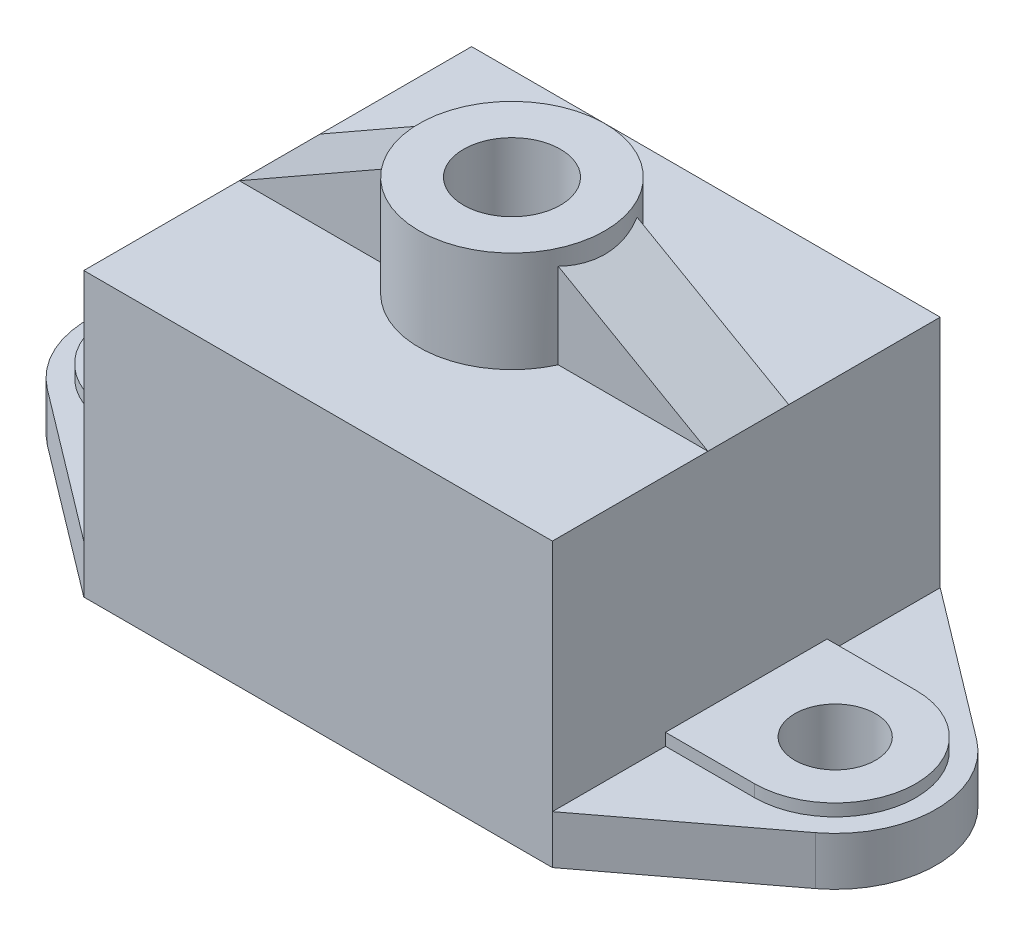
ISO-10303-21;
HEADER;
FILE_DESCRIPTION(('STEP AP214'),'2;1');
FILE_NAME('part.step','',(''),(''),'','','');
FILE_SCHEMA(('AUTOMOTIVE_DESIGN { 1 0 10303 214 1 1 1 1 }'));
ENDSEC;
DATA;
#1=APPLICATION_CONTEXT('core data for automotive mechanical design processes');
#2=APPLICATION_PROTOCOL_DEFINITION('international standard','automotive_design',2000,#1);
#3=PRODUCT_CONTEXT('',#1,'mechanical');
#4=PRODUCT('Part','Part','',(#3));
#5=PRODUCT_RELATED_PRODUCT_CATEGORY('part','',(#4));
#6=PRODUCT_DEFINITION_FORMATION('','',#4);
#7=PRODUCT_DEFINITION_CONTEXT('part definition',#1,'design');
#8=PRODUCT_DEFINITION('design','',#6,#7);
#9=PRODUCT_DEFINITION_SHAPE('','',#8);
#10=(LENGTH_UNIT() NAMED_UNIT(*) SI_UNIT(.MILLI.,.METRE.));
#11=(NAMED_UNIT(*) PLANE_ANGLE_UNIT() SI_UNIT($,.RADIAN.));
#12=(NAMED_UNIT(*) SI_UNIT($,.STERADIAN.) SOLID_ANGLE_UNIT());
#13=UNCERTAINTY_MEASURE_WITH_UNIT(LENGTH_MEASURE(1.E-05),#10,'distance_accuracy_value','');
#14=(GEOMETRIC_REPRESENTATION_CONTEXT(3) GLOBAL_UNCERTAINTY_ASSIGNED_CONTEXT((#13)) GLOBAL_UNIT_ASSIGNED_CONTEXT((#10,
#11,#12)) REPRESENTATION_CONTEXT('',''));
#15=CARTESIAN_POINT('',(0.,0.,0.));
#16=DIRECTION('',(0.,0.,1.));
#17=DIRECTION('',(1.,0.,0.));
#18=AXIS2_PLACEMENT_3D('',#15,#16,#17);
#19=CARTESIAN_POINT('',(116.,70.,96.));
#20=DIRECTION('',(0.,-1.,0.));
#21=DIRECTION('',(0.,0.,-1.));
#22=AXIS2_PLACEMENT_3D('',#19,#20,#21);
#23=PLANE('',#22);
#24=DIRECTION('',(-1.,0.,0.));
#25=VECTOR('',#24,1.);
#26=CARTESIAN_POINT('',(35.,70.,57.5));
#27=LINE('',#26,#25);
#28=CARTESIAN_POINT('',(37.0536399343466,70.,57.5));
#29=VERTEX_POINT('',#28);
#30=CARTESIAN_POINT('',(0.,70.,57.5));
#31=VERTEX_POINT('',#30);
#32=EDGE_CURVE('E208',#29,#31,#27,.T.);
#33=ORIENTED_EDGE('',*,*,#32,.T.);
#34=DIRECTION('',(0.,0.,-1.));
#35=VECTOR('',#34,1.);
#36=CARTESIAN_POINT('',(0.,70.,96.));
#37=LINE('',#36,#35);
#38=CARTESIAN_POINT('',(0.,70.,96.));
#39=VERTEX_POINT('',#38);
#40=EDGE_CURVE('E224',#39,#31,#37,.T.);
#41=ORIENTED_EDGE('',*,*,#40,.F.);
#42=DIRECTION('',(-1.,0.,0.));
#43=VECTOR('',#42,1.);
#44=CARTESIAN_POINT('',(116.,70.,96.));
#45=LINE('',#44,#43);
#46=CARTESIAN_POINT('',(116.,70.,96.));
#47=VERTEX_POINT('',#46);
#48=EDGE_CURVE('E232',#47,#39,#45,.T.);
#49=ORIENTED_EDGE('',*,*,#48,.F.);
#50=DIRECTION('',(0.,0.,-1.));
#51=VECTOR('',#50,1.);
#52=CARTESIAN_POINT('',(116.,70.,96.));
#53=LINE('',#52,#51);
#54=CARTESIAN_POINT('',(116.,70.,57.5));
#55=VERTEX_POINT('',#54);
#56=EDGE_CURVE('E231',#47,#55,#53,.T.);
#57=ORIENTED_EDGE('',*,*,#56,.T.);
#58=DIRECTION('',(1.,0.,0.));
#59=VECTOR('',#58,1.);
#60=CARTESIAN_POINT('',(81.,70.,57.5));
#61=LINE('',#60,#59);
#62=CARTESIAN_POINT('',(78.9463600656534,70.,57.5));
#63=VERTEX_POINT('',#62);
#64=EDGE_CURVE('E259',#63,#55,#61,.T.);
#65=ORIENTED_EDGE('',*,*,#64,.F.);
#66=CARTESIAN_POINT('',(58.,70.,48.));
#67=DIRECTION('',(0.,-1.,0.));
#68=DIRECTION('',(0.,0.,-1.));
#69=AXIS2_PLACEMENT_3D('',#66,#67,#68);
#70=CIRCLE('',#69,23.);
#71=EDGE_CURVE('E228',#29,#63,#70,.F.);
#72=ORIENTED_EDGE('',*,*,#71,.F.);
#73=EDGE_LOOP('',(#33,#41,#49,#57,#65,#72));
#74=FACE_BOUND('',#73,.T.);
#75=ADVANCED_FACE('F41',(#74),#23,.F.);
#76=CARTESIAN_POINT('',(58.,95.,48.));
#77=DIRECTION('',(0.,-1.,0.));
#78=DIRECTION('',(0.,0.,-1.));
#79=AXIS2_PLACEMENT_3D('',#76,#77,#78);
#80=CYLINDRICAL_SURFACE('',#79,23.);
#81=CARTESIAN_POINT('',(58.,95.,48.));
#82=DIRECTION('',(0.,1.,0.));
#83=DIRECTION('',(0.,0.,1.));
#84=AXIS2_PLACEMENT_3D('',#81,#82,#83);
#85=CIRCLE('',#84,23.);
#86=CARTESIAN_POINT('',(58.,95.,71.));
#87=VERTEX_POINT('',#86);
#88=EDGE_CURVE('E277',#87,#87,#85,.T.);
#89=ORIENTED_EDGE('',*,*,#88,.F.);
#90=EDGE_LOOP('',(#89));
#91=FACE_BOUND('',#90,.T.);
#92=DIRECTION('',(0.,-1.,0.));
#93=VECTOR('',#92,1.);
#94=CARTESIAN_POINT('',(37.0536399343466,95.,57.5));
#95=LINE('',#94,#93);
#96=CARTESIAN_POINT('',(37.0536399343466,91.128111029422,57.5));
#97=VERTEX_POINT('',#96);
#98=EDGE_CURVE('E216',#29,#97,#95,.F.);
#99=ORIENTED_EDGE('',*,*,#98,.F.);
#100=ORIENTED_EDGE('',*,*,#71,.T.);
#101=DIRECTION('',(0.,-1.,0.));
#102=VECTOR('',#101,1.);
#103=CARTESIAN_POINT('',(78.9463600656534,95.,57.5));
#104=LINE('',#103,#102);
#105=CARTESIAN_POINT('',(78.9463600656534,91.1281110294221,57.5));
#106=VERTEX_POINT('',#105);
#107=EDGE_CURVE('E11',#106,#63,#104,.T.);
#108=ORIENTED_EDGE('',*,*,#107,.F.);
#109=CARTESIAN_POINT('',(58.,103.071796505762,48.));
#110=DIRECTION('',(-0.495336394229628,-0.868701247007043,0.));
#111=DIRECTION('',(0.868701247007043,-0.495336394229628,0.));
#112=AXIS2_PLACEMENT_3D('',#109,#110,#111);
#113=ELLIPSE('',#112,26.4763059558651,23.);
#114=CARTESIAN_POINT('',(78.4633819296811,91.4035067988981,37.5));
#115=VERTEX_POINT('',#114);
#116=EDGE_CURVE('E47',#115,#106,#113,.T.);
#117=ORIENTED_EDGE('',*,*,#116,.F.);
#118=DIRECTION('',(0.,-1.,0.));
#119=VECTOR('',#118,1.);
#120=CARTESIAN_POINT('',(78.4633819296811,95.,37.5));
#121=LINE('',#120,#119);
#122=CARTESIAN_POINT('',(78.4633819296811,70.,37.5));
#123=VERTEX_POINT('',#122);
#124=EDGE_CURVE('E242',#115,#123,#121,.T.);
#125=ORIENTED_EDGE('',*,*,#124,.T.);
#126=CARTESIAN_POINT('',(37.5366180703189,70.,37.5));
#127=VERTEX_POINT('',#126);
#128=EDGE_CURVE('E241',#123,#127,#70,.F.);
#129=ORIENTED_EDGE('',*,*,#128,.T.);
#130=DIRECTION('',(0.,-1.,0.));
#131=VECTOR('',#130,1.);
#132=CARTESIAN_POINT('',(37.5366180703189,95.,37.5));
#133=LINE('',#132,#131);
#134=CARTESIAN_POINT('',(37.5366180703189,91.403506798898,37.5));
#135=VERTEX_POINT('',#134);
#136=EDGE_CURVE('E209',#127,#135,#133,.F.);
#137=ORIENTED_EDGE('',*,*,#136,.T.);
#138=CARTESIAN_POINT('',(58.,103.071796505762,48.));
#139=DIRECTION('',(-0.495336394229628,0.868701247007043,0.));
#140=DIRECTION('',(-0.868701247007043,-0.495336394229628,0.));
#141=AXIS2_PLACEMENT_3D('',#138,#139,#140);
#142=ELLIPSE('',#141,26.4763059558651,23.);
#143=EDGE_CURVE('E265',#135,#97,#142,.T.);
#144=ORIENTED_EDGE('',*,*,#143,.T.);
#145=EDGE_LOOP('',(#99,#100,#108,#117,#125,#129,#137,#144));
#146=FACE_BOUND('',#145,.T.);
#147=ADVANCED_FACE('F258',(#91,#146),#80,.T.);
#148=CARTESIAN_POINT('',(0.,70.,37.5));
#149=VERTEX_POINT('',#148);
#150=CARTESIAN_POINT('',(0.,70.,0.));
#151=VERTEX_POINT('',#150);
#152=EDGE_CURVE('E233',#149,#151,#37,.T.);
#153=ORIENTED_EDGE('',*,*,#152,.F.);
#154=DIRECTION('',(-1.,0.,0.));
#155=VECTOR('',#154,1.);
#156=CARTESIAN_POINT('',(35.,70.,37.5));
#157=LINE('',#156,#155);
#158=EDGE_CURVE('E220',#127,#149,#157,.T.);
#159=ORIENTED_EDGE('',*,*,#158,.F.);
#160=ORIENTED_EDGE('',*,*,#128,.F.);
#161=DIRECTION('',(1.,0.,0.));
#162=VECTOR('',#161,1.);
#163=CARTESIAN_POINT('',(81.,70.,37.5));
#164=LINE('',#163,#162);
#165=CARTESIAN_POINT('',(116.,70.,37.5));
#166=VERTEX_POINT('',#165);
#167=EDGE_CURVE('E61',#123,#166,#164,.T.);
#168=ORIENTED_EDGE('',*,*,#167,.T.);
#169=CARTESIAN_POINT('',(116.,70.,0.));
#170=VERTEX_POINT('',#169);
#171=EDGE_CURVE('E229',#166,#170,#53,.T.);
#172=ORIENTED_EDGE('',*,*,#171,.T.);
#173=DIRECTION('',(-1.,0.,0.));
#174=VECTOR('',#173,1.);
#175=CARTESIAN_POINT('',(116.,70.,0.));
#176=LINE('',#175,#174);
#177=EDGE_CURVE('E240',#170,#151,#176,.T.);
#178=ORIENTED_EDGE('',*,*,#177,.T.);
#179=EDGE_LOOP('',(#153,#159,#160,#168,#172,#178));
#180=FACE_BOUND('',#179,.T.);
#181=ADVANCED_FACE('F432',(#180),#23,.F.);
#182=CARTESIAN_POINT('',(116.,0.,96.));
#183=DIRECTION('',(-1.,0.,0.));
#184=DIRECTION('',(0.,0.,1.));
#185=AXIS2_PLACEMENT_3D('',#182,#183,#184);
#186=PLANE('',#185);
#187=DIRECTION('',(0.,-1.,0.));
#188=VECTOR('',#187,1.);
#189=CARTESIAN_POINT('',(116.,15.,28.));
#190=LINE('',#189,#188);
#191=CARTESIAN_POINT('',(116.,15.,28.));
#192=VERTEX_POINT('',#191);
#193=CARTESIAN_POINT('',(116.,12.,28.));
#194=VERTEX_POINT('',#193);
#195=EDGE_CURVE('E373',#192,#194,#190,.T.);
#196=ORIENTED_EDGE('',*,*,#195,.T.);
#197=DIRECTION('',(0.,0.,1.));
#198=VECTOR('',#197,1.);
#199=CARTESIAN_POINT('',(116.,12.,0.));
#200=LINE('',#199,#198);
#201=CARTESIAN_POINT('',(116.,12.,0.));
#202=VERTEX_POINT('',#201);
#203=EDGE_CURVE('E390',#202,#194,#200,.T.);
#204=ORIENTED_EDGE('',*,*,#203,.F.);
#205=DIRECTION('',(0.,1.,0.));
#206=VECTOR('',#205,1.);
#207=CARTESIAN_POINT('',(116.,0.,0.));
#208=LINE('',#207,#206);
#209=EDGE_CURVE('E416',#202,#170,#208,.T.);
#210=ORIENTED_EDGE('',*,*,#209,.T.);
#211=ORIENTED_EDGE('',*,*,#171,.F.);
#212=DIRECTION('',(0.,0.,-1.));
#213=VECTOR('',#212,1.);
#214=CARTESIAN_POINT('',(116.,70.,57.5));
#215=LINE('',#214,#213);
#216=EDGE_CURVE('E269',#55,#166,#215,.T.);
#217=ORIENTED_EDGE('',*,*,#216,.F.);
#218=ORIENTED_EDGE('',*,*,#56,.F.);
#219=DIRECTION('',(0.,1.,0.));
#220=VECTOR('',#219,1.);
#221=CARTESIAN_POINT('',(116.,0.,96.));
#222=LINE('',#221,#220);
#223=CARTESIAN_POINT('',(116.,12.,96.));
#224=VERTEX_POINT('',#223);
#225=EDGE_CURVE('E409',#224,#47,#222,.T.);
#226=ORIENTED_EDGE('',*,*,#225,.F.);
#227=CARTESIAN_POINT('',(116.,12.,68.));
#228=VERTEX_POINT('',#227);
#229=EDGE_CURVE('E387',#228,#224,#200,.T.);
#230=ORIENTED_EDGE('',*,*,#229,.F.);
#231=DIRECTION('',(0.,-1.,0.));
#232=VECTOR('',#231,1.);
#233=CARTESIAN_POINT('',(116.,15.,68.));
#234=LINE('',#233,#232);
#235=CARTESIAN_POINT('',(116.,15.,68.));
#236=VERTEX_POINT('',#235);
#237=EDGE_CURVE('E371',#236,#228,#234,.T.);
#238=ORIENTED_EDGE('',*,*,#237,.F.);
#239=DIRECTION('',(0.,0.,1.));
#240=VECTOR('',#239,1.);
#241=CARTESIAN_POINT('',(116.,15.,28.));
#242=LINE('',#241,#240);
#243=EDGE_CURVE('E360',#192,#236,#242,.T.);
#244=ORIENTED_EDGE('',*,*,#243,.F.);
#245=EDGE_LOOP('',(#196,#204,#210,#211,#217,#218,#226,#230,#238,#244));
#246=FACE_BOUND('',#245,.T.);
#247=ADVANCED_FACE('F430',(#246),#186,.F.);
#248=CARTESIAN_POINT('',(138.,12.,48.));
#249=DIRECTION('',(0.,1.,0.));
#250=DIRECTION('',(0.,0.,1.));
#251=AXIS2_PLACEMENT_3D('',#248,#249,#250);
#252=PLANE('',#251);
#253=ORIENTED_EDGE('',*,*,#203,.T.);
#254=DIRECTION('',(-1.,0.,0.));
#255=VECTOR('',#254,1.);
#256=CARTESIAN_POINT('',(138.,12.,28.));
#257=LINE('',#256,#255);
#258=CARTESIAN_POINT('',(138.,12.,28.));
#259=VERTEX_POINT('',#258);
#260=EDGE_CURVE('E366',#259,#194,#257,.T.);
#261=ORIENTED_EDGE('',*,*,#260,.F.);
#262=CARTESIAN_POINT('',(138.,12.,48.));
#263=DIRECTION('',(0.,1.,0.));
#264=DIRECTION('',(0.,0.,1.));
#265=AXIS2_PLACEMENT_3D('',#262,#263,#264);
#266=CIRCLE('',#265,20.);
#267=CARTESIAN_POINT('',(138.,12.,68.));
#268=VERTEX_POINT('',#267);
#269=EDGE_CURVE('E349',#268,#259,#266,.T.);
#270=ORIENTED_EDGE('',*,*,#269,.F.);
#271=DIRECTION('',(1.,0.,0.));
#272=VECTOR('',#271,1.);
#273=CARTESIAN_POINT('',(116.,12.,68.));
#274=LINE('',#273,#272);
#275=EDGE_CURVE('E357',#228,#268,#274,.T.);
#276=ORIENTED_EDGE('',*,*,#275,.F.);
#277=ORIENTED_EDGE('',*,*,#229,.T.);
#278=DIRECTION('',(0.797409398842377,0.,-0.603438688383367));
#279=VECTOR('',#278,1.);
#280=CARTESIAN_POINT('',(116.,12.,96.));
#281=LINE('',#280,#279);
#282=CARTESIAN_POINT('',(153.085967209584,12.,67.9352349710594));
#283=VERTEX_POINT('',#282);
#284=EDGE_CURVE('E388',#224,#283,#281,.T.);
#285=ORIENTED_EDGE('',*,*,#284,.T.);
#286=CARTESIAN_POINT('',(138.,12.,48.));
#287=DIRECTION('',(0.,1.,0.));
#288=DIRECTION('',(0.,0.,1.));
#289=AXIS2_PLACEMENT_3D('',#286,#287,#288);
#290=CIRCLE('',#289,25.);
#291=CARTESIAN_POINT('',(153.085967209584,12.,28.0647650289406));
#292=VERTEX_POINT('',#291);
#293=EDGE_CURVE('E378',#283,#292,#290,.T.);
#294=ORIENTED_EDGE('',*,*,#293,.T.);
#295=DIRECTION('',(-0.797409398842377,0.,-0.603438688383367));
#296=VECTOR('',#295,1.);
#297=CARTESIAN_POINT('',(116.,12.,0.));
#298=LINE('',#297,#296);
#299=EDGE_CURVE('E385',#292,#202,#298,.T.);
#300=ORIENTED_EDGE('',*,*,#299,.T.);
#301=EDGE_LOOP('',(#253,#261,#270,#276,#277,#285,#294,#300));
#302=FACE_BOUND('',#301,.T.);
#303=ADVANCED_FACE('F463',(#302),#252,.T.);
#304=CARTESIAN_POINT('',(0.,70.,96.));
#305=DIRECTION('',(1.,0.,0.));
#306=DIRECTION('',(0.,0.,-1.));
#307=AXIS2_PLACEMENT_3D('',#304,#305,#306);
#308=PLANE('',#307);
#309=DIRECTION('',(0.,0.,1.));
#310=VECTOR('',#309,1.);
#311=CARTESIAN_POINT('',(0.,15.,28.));
#312=LINE('',#311,#310);
#313=CARTESIAN_POINT('',(0.,15.,28.));
#314=VERTEX_POINT('',#313);
#315=CARTESIAN_POINT('',(0.,15.,68.));
#316=VERTEX_POINT('',#315);
#317=EDGE_CURVE('E294',#314,#316,#312,.T.);
#318=ORIENTED_EDGE('',*,*,#317,.T.);
#319=DIRECTION('',(0.,-1.,0.));
#320=VECTOR('',#319,1.);
#321=CARTESIAN_POINT('',(0.,15.,68.));
#322=LINE('',#321,#320);
#323=CARTESIAN_POINT('',(0.,12.,68.));
#324=VERTEX_POINT('',#323);
#325=EDGE_CURVE('E309',#316,#324,#322,.T.);
#326=ORIENTED_EDGE('',*,*,#325,.T.);
#327=DIRECTION('',(0.,0.,1.));
#328=VECTOR('',#327,1.);
#329=CARTESIAN_POINT('',(0.,12.,0.));
#330=LINE('',#329,#328);
#331=CARTESIAN_POINT('',(0.,12.,96.));
#332=VERTEX_POINT('',#331);
#333=EDGE_CURVE('E324',#324,#332,#330,.T.);
#334=ORIENTED_EDGE('',*,*,#333,.T.);
#335=DIRECTION('',(0.,-1.,0.));
#336=VECTOR('',#335,1.);
#337=CARTESIAN_POINT('',(0.,70.,96.));
#338=LINE('',#337,#336);
#339=EDGE_CURVE('E230',#39,#332,#338,.T.);
#340=ORIENTED_EDGE('',*,*,#339,.F.);
#341=ORIENTED_EDGE('',*,*,#40,.T.);
#342=DIRECTION('',(0.,0.,-1.));
#343=VECTOR('',#342,1.);
#344=CARTESIAN_POINT('',(0.,70.,57.5));
#345=LINE('',#344,#343);
#346=EDGE_CURVE('E202',#31,#149,#345,.T.);
#347=ORIENTED_EDGE('',*,*,#346,.T.);
#348=ORIENTED_EDGE('',*,*,#152,.T.);
#349=DIRECTION('',(0.,-1.,0.));
#350=VECTOR('',#349,1.);
#351=CARTESIAN_POINT('',(0.,70.,0.));
#352=LINE('',#351,#350);
#353=CARTESIAN_POINT('',(0.,12.,0.));
#354=VERTEX_POINT('',#353);
#355=EDGE_CURVE('E404',#151,#354,#352,.T.);
#356=ORIENTED_EDGE('',*,*,#355,.T.);
#357=CARTESIAN_POINT('',(0.,12.,28.));
#358=VERTEX_POINT('',#357);
#359=EDGE_CURVE('E321',#354,#358,#330,.T.);
#360=ORIENTED_EDGE('',*,*,#359,.T.);
#361=DIRECTION('',(0.,-1.,0.));
#362=VECTOR('',#361,1.);
#363=CARTESIAN_POINT('',(0.,15.,28.));
#364=LINE('',#363,#362);
#365=EDGE_CURVE('E310',#314,#358,#364,.T.);
#366=ORIENTED_EDGE('',*,*,#365,.F.);
#367=EDGE_LOOP('',(#318,#326,#334,#340,#341,#347,#348,#356,#360,#366));
#368=FACE_BOUND('',#367,.T.);
#369=ADVANCED_FACE('F43',(#368),#308,.F.);
#370=CARTESIAN_POINT('',(0.,0.,96.));
#371=DIRECTION('',(0.,1.,0.));
#372=DIRECTION('',(0.,0.,1.));
#373=AXIS2_PLACEMENT_3D('',#370,#371,#372);
#374=PLANE('',#373);
#375=CARTESIAN_POINT('',(-22.,0.,48.));
#376=DIRECTION('',(0.,-1.,0.));
#377=DIRECTION('',(0.,0.,1.));
#378=AXIS2_PLACEMENT_3D('',#375,#376,#377);
#379=CIRCLE('',#378,10.);
#380=CARTESIAN_POINT('',(-22.,0.,58.));
#381=VERTEX_POINT('',#380);
#382=EDGE_CURVE('E285',#381,#381,#379,.T.);
#383=ORIENTED_EDGE('',*,*,#382,.F.);
#384=EDGE_LOOP('',(#383));
#385=FACE_BOUND('',#384,.T.);
#386=CARTESIAN_POINT('',(138.,0.,48.));
#387=DIRECTION('',(0.,1.,0.));
#388=DIRECTION('',(0.,0.,1.));
#389=AXIS2_PLACEMENT_3D('',#386,#387,#388);
#390=CIRCLE('',#389,10.);
#391=CARTESIAN_POINT('',(138.,0.,58.));
#392=VERTEX_POINT('',#391);
#393=EDGE_CURVE('E350',#392,#392,#390,.T.);
#394=ORIENTED_EDGE('',*,*,#393,.T.);
#395=EDGE_LOOP('',(#394));
#396=FACE_BOUND('',#395,.T.);
#397=DIRECTION('',(1.,0.,0.));
#398=VECTOR('',#397,1.);
#399=CARTESIAN_POINT('',(0.,0.,0.));
#400=LINE('',#399,#398);
#401=CARTESIAN_POINT('',(0.,0.,0.));
#402=VERTEX_POINT('',#401);
#403=CARTESIAN_POINT('',(116.,0.,0.));
#404=VERTEX_POINT('',#403);
#405=EDGE_CURVE('E414',#402,#404,#400,.T.);
#406=ORIENTED_EDGE('',*,*,#405,.T.);
#407=DIRECTION('',(-0.797409398842377,0.,-0.603438688383367));
#408=VECTOR('',#407,1.);
#409=CARTESIAN_POINT('',(116.,0.,0.));
#410=LINE('',#409,#408);
#411=CARTESIAN_POINT('',(153.085967209584,0.,28.0647650289406));
#412=VERTEX_POINT('',#411);
#413=EDGE_CURVE('E394',#412,#404,#410,.T.);
#414=ORIENTED_EDGE('',*,*,#413,.F.);
#415=CARTESIAN_POINT('',(138.,0.,48.));
#416=DIRECTION('',(0.,1.,0.));
#417=DIRECTION('',(0.,0.,1.));
#418=AXIS2_PLACEMENT_3D('',#415,#416,#417);
#419=CIRCLE('',#418,25.);
#420=CARTESIAN_POINT('',(153.085967209584,0.,67.9352349710594));
#421=VERTEX_POINT('',#420);
#422=EDGE_CURVE('E377',#421,#412,#419,.T.);
#423=ORIENTED_EDGE('',*,*,#422,.F.);
#424=DIRECTION('',(0.797409398842377,0.,-0.603438688383367));
#425=VECTOR('',#424,1.);
#426=CARTESIAN_POINT('',(116.,0.,96.));
#427=LINE('',#426,#425);
#428=CARTESIAN_POINT('',(116.,0.,96.));
#429=VERTEX_POINT('',#428);
#430=EDGE_CURVE('E384',#429,#421,#427,.T.);
#431=ORIENTED_EDGE('',*,*,#430,.F.);
#432=DIRECTION('',(1.,0.,0.));
#433=VECTOR('',#432,1.);
#434=CARTESIAN_POINT('',(0.,0.,96.));
#435=LINE('',#434,#433);
#436=CARTESIAN_POINT('',(0.,0.,96.));
#437=VERTEX_POINT('',#436);
#438=EDGE_CURVE('E407',#437,#429,#435,.T.);
#439=ORIENTED_EDGE('',*,*,#438,.F.);
#440=DIRECTION('',(-0.797409398842377,0.,-0.603438688383367));
#441=VECTOR('',#440,1.);
#442=CARTESIAN_POINT('',(0.,0.,96.));
#443=LINE('',#442,#441);
#444=CARTESIAN_POINT('',(-37.0859672095842,0.,67.9352349710594));
#445=VERTEX_POINT('',#444);
#446=EDGE_CURVE('E334',#437,#445,#443,.T.);
#447=ORIENTED_EDGE('',*,*,#446,.T.);
#448=CARTESIAN_POINT('',(-22.,0.,48.));
#449=DIRECTION('',(0.,-1.,0.));
#450=DIRECTION('',(0.,0.,1.));
#451=AXIS2_PLACEMENT_3D('',#448,#449,#450);
#452=CIRCLE('',#451,25.);
#453=CARTESIAN_POINT('',(-37.0859672095842,0.,28.0647650289406));
#454=VERTEX_POINT('',#453);
#455=EDGE_CURVE('E314',#445,#454,#452,.T.);
#456=ORIENTED_EDGE('',*,*,#455,.T.);
#457=DIRECTION('',(0.797409398842377,0.,-0.603438688383367));
#458=VECTOR('',#457,1.);
#459=CARTESIAN_POINT('',(0.,0.,0.));
#460=LINE('',#459,#458);
#461=EDGE_CURVE('E318',#454,#402,#460,.T.);
#462=ORIENTED_EDGE('',*,*,#461,.T.);
#463=EDGE_LOOP('',(#406,#414,#423,#431,#439,#447,#456,#462));
#464=FACE_BOUND('',#463,.T.);
#465=ADVANCED_FACE('F468',(#385,#396,#464),#374,.F.);
#466=CARTESIAN_POINT('',(0.,0.,96.));
#467=DIRECTION('',(0.,0.,1.));
#468=DIRECTION('',(1.,0.,0.));
#469=AXIS2_PLACEMENT_3D('',#466,#467,#468);
#470=PLANE('',#469);
#471=ORIENTED_EDGE('',*,*,#339,.T.);
#472=DIRECTION('',(0.,-1.,0.));
#473=VECTOR('',#472,1.);
#474=CARTESIAN_POINT('',(0.,12.,96.));
#475=LINE('',#474,#473);
#476=EDGE_CURVE('E342',#332,#437,#475,.T.);
#477=ORIENTED_EDGE('',*,*,#476,.T.);
#478=ORIENTED_EDGE('',*,*,#438,.T.);
#479=EDGE_CURVE('E406',#429,#224,#222,.T.);
#480=ORIENTED_EDGE('',*,*,#479,.T.);
#481=ORIENTED_EDGE('',*,*,#225,.T.);
#482=ORIENTED_EDGE('',*,*,#48,.T.);
#483=EDGE_LOOP('',(#471,#477,#478,#480,#481,#482));
#484=FACE_BOUND('',#483,.T.);
#485=ADVANCED_FACE('F475',(#484),#470,.T.);
#486=CARTESIAN_POINT('',(0.,0.,0.));
#487=DIRECTION('',(0.,0.,1.));
#488=DIRECTION('',(1.,0.,0.));
#489=AXIS2_PLACEMENT_3D('',#486,#487,#488);
#490=PLANE('',#489);
#491=ORIENTED_EDGE('',*,*,#355,.F.);
#492=ORIENTED_EDGE('',*,*,#177,.F.);
#493=ORIENTED_EDGE('',*,*,#209,.F.);
#494=EDGE_CURVE('E417',#404,#202,#208,.T.);
#495=ORIENTED_EDGE('',*,*,#494,.F.);
#496=ORIENTED_EDGE('',*,*,#405,.F.);
#497=DIRECTION('',(0.,-1.,0.));
#498=VECTOR('',#497,1.);
#499=CARTESIAN_POINT('',(0.,12.,0.));
#500=LINE('',#499,#498);
#501=EDGE_CURVE('E339',#354,#402,#500,.T.);
#502=ORIENTED_EDGE('',*,*,#501,.F.);
#503=EDGE_LOOP('',(#491,#492,#493,#495,#496,#502));
#504=FACE_BOUND('',#503,.T.);
#505=ADVANCED_FACE('F427',(#504),#490,.F.);
#506=CARTESIAN_POINT('',(138.,12.,48.));
#507=DIRECTION('',(0.,-1.,0.));
#508=DIRECTION('',(0.,0.,-1.));
#509=AXIS2_PLACEMENT_3D('',#506,#507,#508);
#510=CYLINDRICAL_SURFACE('',#509,25.);
#511=ORIENTED_EDGE('',*,*,#422,.T.);
#512=DIRECTION('',(0.,-1.,0.));
#513=VECTOR('',#512,1.);
#514=CARTESIAN_POINT('',(153.085967209584,12.,28.0647650289406));
#515=LINE('',#514,#513);
#516=EDGE_CURVE('E402',#292,#412,#515,.T.);
#517=ORIENTED_EDGE('',*,*,#516,.F.);
#518=ORIENTED_EDGE('',*,*,#293,.F.);
#519=DIRECTION('',(0.,-1.,0.));
#520=VECTOR('',#519,1.);
#521=CARTESIAN_POINT('',(153.085967209584,12.,67.9352349710594));
#522=LINE('',#521,#520);
#523=EDGE_CURVE('E395',#283,#421,#522,.T.);
#524=ORIENTED_EDGE('',*,*,#523,.T.);
#525=EDGE_LOOP('',(#511,#517,#518,#524));
#526=FACE_BOUND('',#525,.T.);
#527=ADVANCED_FACE('F493',(#526),#510,.T.);
#528=CARTESIAN_POINT('',(116.,12.,0.));
#529=DIRECTION('',(-0.603438688383367,0.,0.797409398842377));
#530=DIRECTION('',(0.797409398842377,0.,0.603438688383367));
#531=AXIS2_PLACEMENT_3D('',#528,#529,#530);
#532=PLANE('',#531);
#533=ORIENTED_EDGE('',*,*,#413,.T.);
#534=ORIENTED_EDGE('',*,*,#494,.T.);
#535=ORIENTED_EDGE('',*,*,#299,.F.);
#536=ORIENTED_EDGE('',*,*,#516,.T.);
#537=EDGE_LOOP('',(#533,#534,#535,#536));
#538=FACE_BOUND('',#537,.T.);
#539=ADVANCED_FACE('F487',(#538),#532,.F.);
#540=CARTESIAN_POINT('',(116.,12.,96.));
#541=DIRECTION('',(-0.603438688383367,0.,-0.797409398842377));
#542=DIRECTION('',(-0.797409398842377,0.,0.603438688383367));
#543=AXIS2_PLACEMENT_3D('',#540,#541,#542);
#544=PLANE('',#543);
#545=ORIENTED_EDGE('',*,*,#430,.T.);
#546=ORIENTED_EDGE('',*,*,#523,.F.);
#547=ORIENTED_EDGE('',*,*,#284,.F.);
#548=ORIENTED_EDGE('',*,*,#479,.F.);
#549=EDGE_LOOP('',(#545,#546,#547,#548));
#550=FACE_BOUND('',#549,.T.);
#551=ADVANCED_FACE('F500',(#550),#544,.F.);
#552=CARTESIAN_POINT('',(138.,15.,48.));
#553=DIRECTION('',(0.,-1.,0.));
#554=DIRECTION('',(0.,0.,-1.));
#555=AXIS2_PLACEMENT_3D('',#552,#553,#554);
#556=CYLINDRICAL_SURFACE('',#555,20.);
#557=ORIENTED_EDGE('',*,*,#269,.T.);
#558=DIRECTION('',(0.,-1.,0.));
#559=VECTOR('',#558,1.);
#560=CARTESIAN_POINT('',(138.,15.,28.));
#561=LINE('',#560,#559);
#562=CARTESIAN_POINT('',(138.,15.,28.));
#563=VERTEX_POINT('',#562);
#564=EDGE_CURVE('E376',#563,#259,#561,.T.);
#565=ORIENTED_EDGE('',*,*,#564,.F.);
#566=CARTESIAN_POINT('',(138.,15.,48.));
#567=DIRECTION('',(0.,1.,0.));
#568=DIRECTION('',(0.,0.,1.));
#569=AXIS2_PLACEMENT_3D('',#566,#567,#568);
#570=CIRCLE('',#569,20.);
#571=CARTESIAN_POINT('',(138.,15.,68.));
#572=VERTEX_POINT('',#571);
#573=EDGE_CURVE('E354',#572,#563,#570,.T.);
#574=ORIENTED_EDGE('',*,*,#573,.F.);
#575=DIRECTION('',(0.,-1.,0.));
#576=VECTOR('',#575,1.);
#577=CARTESIAN_POINT('',(138.,15.,68.));
#578=LINE('',#577,#576);
#579=EDGE_CURVE('E361',#572,#268,#578,.T.);
#580=ORIENTED_EDGE('',*,*,#579,.T.);
#581=EDGE_LOOP('',(#557,#565,#574,#580));
#582=FACE_BOUND('',#581,.T.);
#583=ADVANCED_FACE('F555',(#582),#556,.T.);
#584=CARTESIAN_POINT('',(138.,15.,28.));
#585=DIRECTION('',(0.,0.,1.));
#586=DIRECTION('',(1.,0.,0.));
#587=AXIS2_PLACEMENT_3D('',#584,#585,#586);
#588=PLANE('',#587);
#589=ORIENTED_EDGE('',*,*,#260,.T.);
#590=ORIENTED_EDGE('',*,*,#195,.F.);
#591=DIRECTION('',(-1.,0.,0.));
#592=VECTOR('',#591,1.);
#593=CARTESIAN_POINT('',(138.,15.,28.));
#594=LINE('',#593,#592);
#595=EDGE_CURVE('E358',#563,#192,#594,.T.);
#596=ORIENTED_EDGE('',*,*,#595,.F.);
#597=ORIENTED_EDGE('',*,*,#564,.T.);
#598=EDGE_LOOP('',(#589,#590,#596,#597));
#599=FACE_BOUND('',#598,.T.);
#600=ADVANCED_FACE('F550',(#599),#588,.F.);
#601=CARTESIAN_POINT('',(116.,15.,68.));
#602=DIRECTION('',(0.,0.,-1.));
#603=DIRECTION('',(-1.,0.,0.));
#604=AXIS2_PLACEMENT_3D('',#601,#602,#603);
#605=PLANE('',#604);
#606=ORIENTED_EDGE('',*,*,#275,.T.);
#607=ORIENTED_EDGE('',*,*,#579,.F.);
#608=DIRECTION('',(1.,0.,0.));
#609=VECTOR('',#608,1.);
#610=CARTESIAN_POINT('',(116.,15.,68.));
#611=LINE('',#610,#609);
#612=EDGE_CURVE('E363',#236,#572,#611,.T.);
#613=ORIENTED_EDGE('',*,*,#612,.F.);
#614=ORIENTED_EDGE('',*,*,#237,.T.);
#615=EDGE_LOOP('',(#606,#607,#613,#614));
#616=FACE_BOUND('',#615,.T.);
#617=ADVANCED_FACE('F546',(#616),#605,.F.);
#618=CARTESIAN_POINT('',(138.,15.,48.));
#619=DIRECTION('',(0.,1.,0.));
#620=DIRECTION('',(0.,0.,1.));
#621=AXIS2_PLACEMENT_3D('',#618,#619,#620);
#622=PLANE('',#621);
#623=CARTESIAN_POINT('',(138.,15.,48.));
#624=DIRECTION('',(0.,1.,0.));
#625=DIRECTION('',(0.,0.,1.));
#626=AXIS2_PLACEMENT_3D('',#623,#624,#625);
#627=CIRCLE('',#626,10.);
#628=CARTESIAN_POINT('',(138.,15.,58.));
#629=VERTEX_POINT('',#628);
#630=EDGE_CURVE('E346',#629,#629,#627,.T.);
#631=ORIENTED_EDGE('',*,*,#630,.F.);
#632=EDGE_LOOP('',(#631));
#633=FACE_BOUND('',#632,.T.);
#634=ORIENTED_EDGE('',*,*,#573,.T.);
#635=ORIENTED_EDGE('',*,*,#595,.T.);
#636=ORIENTED_EDGE('',*,*,#243,.T.);
#637=ORIENTED_EDGE('',*,*,#612,.T.);
#638=EDGE_LOOP('',(#634,#635,#636,#637));
#639=FACE_BOUND('',#638,.T.);
#640=ADVANCED_FACE('F536',(#633,#639),#622,.T.);
#641=CARTESIAN_POINT('',(138.,0.,48.));
#642=DIRECTION('',(0.,1.,0.));
#643=DIRECTION('',(0.,0.,1.));
#644=AXIS2_PLACEMENT_3D('',#641,#642,#643);
#645=CYLINDRICAL_SURFACE('',#644,10.);
#646=ORIENTED_EDGE('',*,*,#393,.F.);
#647=EDGE_LOOP('',(#646));
#648=FACE_BOUND('',#647,.T.);
#649=ORIENTED_EDGE('',*,*,#630,.T.);
#650=EDGE_LOOP('',(#649));
#651=FACE_BOUND('',#650,.T.);
#652=ADVANCED_FACE('F535',(#648,#651),#645,.F.);
#653=CARTESIAN_POINT('',(-22.,12.,48.));
#654=DIRECTION('',(0.,-1.,0.));
#655=DIRECTION('',(0.,0.,-1.));
#656=AXIS2_PLACEMENT_3D('',#653,#654,#655);
#657=CYLINDRICAL_SURFACE('',#656,25.);
#658=ORIENTED_EDGE('',*,*,#455,.F.);
#659=DIRECTION('',(0.,-1.,0.));
#660=VECTOR('',#659,1.);
#661=CARTESIAN_POINT('',(-37.0859672095842,12.,67.9352349710594));
#662=LINE('',#661,#660);
#663=CARTESIAN_POINT('',(-37.0859672095842,12.,67.9352349710594));
#664=VERTEX_POINT('',#663);
#665=EDGE_CURVE('E341',#664,#445,#662,.T.);
#666=ORIENTED_EDGE('',*,*,#665,.F.);
#667=CARTESIAN_POINT('',(-22.,12.,48.));
#668=DIRECTION('',(0.,-1.,0.));
#669=DIRECTION('',(0.,0.,1.));
#670=AXIS2_PLACEMENT_3D('',#667,#668,#669);
#671=CIRCLE('',#670,25.);
#672=CARTESIAN_POINT('',(-37.0859672095842,12.,28.0647650289406));
#673=VERTEX_POINT('',#672);
#674=EDGE_CURVE('E317',#664,#673,#671,.T.);
#675=ORIENTED_EDGE('',*,*,#674,.T.);
#676=DIRECTION('',(0.,-1.,0.));
#677=VECTOR('',#676,1.);
#678=CARTESIAN_POINT('',(-37.0859672095842,12.,28.0647650289406));
#679=LINE('',#678,#677);
#680=EDGE_CURVE('E329',#673,#454,#679,.T.);
#681=ORIENTED_EDGE('',*,*,#680,.T.);
#682=EDGE_LOOP('',(#658,#666,#675,#681));
#683=FACE_BOUND('',#682,.T.);
#684=ADVANCED_FACE('F530',(#683),#657,.T.);
#685=CARTESIAN_POINT('',(0.,12.,96.));
#686=DIRECTION('',(-0.603438688383367,0.,0.797409398842377));
#687=DIRECTION('',(0.797409398842377,0.,0.603438688383367));
#688=AXIS2_PLACEMENT_3D('',#685,#686,#687);
#689=PLANE('',#688);
#690=ORIENTED_EDGE('',*,*,#446,.F.);
#691=ORIENTED_EDGE('',*,*,#476,.F.);
#692=DIRECTION('',(-0.797409398842377,0.,-0.603438688383367));
#693=VECTOR('',#692,1.);
#694=CARTESIAN_POINT('',(0.,12.,96.));
#695=LINE('',#694,#693);
#696=EDGE_CURVE('E316',#332,#664,#695,.T.);
#697=ORIENTED_EDGE('',*,*,#696,.T.);
#698=ORIENTED_EDGE('',*,*,#665,.T.);
#699=EDGE_LOOP('',(#690,#691,#697,#698));
#700=FACE_BOUND('',#699,.T.);
#701=ADVANCED_FACE('F504',(#700),#689,.T.);
#702=CARTESIAN_POINT('',(0.,12.,0.));
#703=DIRECTION('',(-0.603438688383367,0.,-0.797409398842377));
#704=DIRECTION('',(-0.797409398842377,0.,0.603438688383367));
#705=AXIS2_PLACEMENT_3D('',#702,#703,#704);
#706=PLANE('',#705);
#707=ORIENTED_EDGE('',*,*,#461,.F.);
#708=ORIENTED_EDGE('',*,*,#680,.F.);
#709=DIRECTION('',(0.797409398842377,0.,-0.603438688383367));
#710=VECTOR('',#709,1.);
#711=CARTESIAN_POINT('',(0.,12.,0.));
#712=LINE('',#711,#710);
#713=EDGE_CURVE('E330',#673,#354,#712,.T.);
#714=ORIENTED_EDGE('',*,*,#713,.T.);
#715=ORIENTED_EDGE('',*,*,#501,.T.);
#716=EDGE_LOOP('',(#707,#708,#714,#715));
#717=FACE_BOUND('',#716,.T.);
#718=ADVANCED_FACE('F509',(#717),#706,.T.);
#719=CARTESIAN_POINT('',(-22.,12.,48.));
#720=DIRECTION('',(0.,1.,0.));
#721=DIRECTION('',(0.,0.,1.));
#722=AXIS2_PLACEMENT_3D('',#719,#720,#721);
#723=PLANE('',#722);
#724=DIRECTION('',(-1.,0.,0.));
#725=VECTOR('',#724,1.);
#726=CARTESIAN_POINT('',(0.,12.,68.));
#727=LINE('',#726,#725);
#728=CARTESIAN_POINT('',(-22.,12.,68.));
#729=VERTEX_POINT('',#728);
#730=EDGE_CURVE('E305',#324,#729,#727,.T.);
#731=ORIENTED_EDGE('',*,*,#730,.T.);
#732=CARTESIAN_POINT('',(-22.,12.,48.));
#733=DIRECTION('',(0.,-1.,0.));
#734=DIRECTION('',(0.,0.,1.));
#735=AXIS2_PLACEMENT_3D('',#732,#733,#734);
#736=CIRCLE('',#735,20.);
#737=CARTESIAN_POINT('',(-22.,12.,28.));
#738=VERTEX_POINT('',#737);
#739=EDGE_CURVE('E284',#729,#738,#736,.T.);
#740=ORIENTED_EDGE('',*,*,#739,.T.);
#741=DIRECTION('',(1.,0.,0.));
#742=VECTOR('',#741,1.);
#743=CARTESIAN_POINT('',(-22.,12.,28.));
#744=LINE('',#743,#742);
#745=EDGE_CURVE('E292',#738,#358,#744,.T.);
#746=ORIENTED_EDGE('',*,*,#745,.T.);
#747=ORIENTED_EDGE('',*,*,#359,.F.);
#748=ORIENTED_EDGE('',*,*,#713,.F.);
#749=ORIENTED_EDGE('',*,*,#674,.F.);
#750=ORIENTED_EDGE('',*,*,#696,.F.);
#751=ORIENTED_EDGE('',*,*,#333,.F.);
#752=EDGE_LOOP('',(#731,#740,#746,#747,#748,#749,#750,#751));
#753=FACE_BOUND('',#752,.T.);
#754=ADVANCED_FACE('F529',(#753),#723,.T.);
#755=CARTESIAN_POINT('',(-22.,15.,48.));
#756=DIRECTION('',(0.,-1.,0.));
#757=DIRECTION('',(0.,0.,-1.));
#758=AXIS2_PLACEMENT_3D('',#755,#756,#757);
#759=CYLINDRICAL_SURFACE('',#758,20.);
#760=ORIENTED_EDGE('',*,*,#739,.F.);
#761=DIRECTION('',(0.,-1.,0.));
#762=VECTOR('',#761,1.);
#763=CARTESIAN_POINT('',(-22.,15.,68.));
#764=LINE('',#763,#762);
#765=CARTESIAN_POINT('',(-22.,15.,68.));
#766=VERTEX_POINT('',#765);
#767=EDGE_CURVE('E315',#766,#729,#764,.T.);
#768=ORIENTED_EDGE('',*,*,#767,.F.);
#769=CARTESIAN_POINT('',(-22.,15.,48.));
#770=DIRECTION('',(0.,-1.,0.));
#771=DIRECTION('',(0.,0.,1.));
#772=AXIS2_PLACEMENT_3D('',#769,#770,#771);
#773=CIRCLE('',#772,20.);
#774=CARTESIAN_POINT('',(-22.,15.,28.));
#775=VERTEX_POINT('',#774);
#776=EDGE_CURVE('E289',#766,#775,#773,.T.);
#777=ORIENTED_EDGE('',*,*,#776,.T.);
#778=DIRECTION('',(0.,-1.,0.));
#779=VECTOR('',#778,1.);
#780=CARTESIAN_POINT('',(-22.,15.,28.));
#781=LINE('',#780,#779);
#782=EDGE_CURVE('E297',#775,#738,#781,.T.);
#783=ORIENTED_EDGE('',*,*,#782,.T.);
#784=EDGE_LOOP('',(#760,#768,#777,#783));
#785=FACE_BOUND('',#784,.T.);
#786=ADVANCED_FACE('F696',(#785),#759,.T.);
#787=CARTESIAN_POINT('',(0.,15.,68.));
#788=DIRECTION('',(0.,0.,1.));
#789=DIRECTION('',(1.,0.,0.));
#790=AXIS2_PLACEMENT_3D('',#787,#788,#789);
#791=PLANE('',#790);
#792=ORIENTED_EDGE('',*,*,#730,.F.);
#793=ORIENTED_EDGE('',*,*,#325,.F.);
#794=DIRECTION('',(-1.,0.,0.));
#795=VECTOR('',#794,1.);
#796=CARTESIAN_POINT('',(0.,15.,68.));
#797=LINE('',#796,#795);
#798=EDGE_CURVE('E293',#316,#766,#797,.T.);
#799=ORIENTED_EDGE('',*,*,#798,.T.);
#800=ORIENTED_EDGE('',*,*,#767,.T.);
#801=EDGE_LOOP('',(#792,#793,#799,#800));
#802=FACE_BOUND('',#801,.T.);
#803=ADVANCED_FACE('F526',(#802),#791,.T.);
#804=CARTESIAN_POINT('',(-22.,15.,28.));
#805=DIRECTION('',(0.,0.,-1.));
#806=DIRECTION('',(-1.,0.,0.));
#807=AXIS2_PLACEMENT_3D('',#804,#805,#806);
#808=PLANE('',#807);
#809=ORIENTED_EDGE('',*,*,#745,.F.);
#810=ORIENTED_EDGE('',*,*,#782,.F.);
#811=DIRECTION('',(1.,0.,0.));
#812=VECTOR('',#811,1.);
#813=CARTESIAN_POINT('',(-22.,15.,28.));
#814=LINE('',#813,#812);
#815=EDGE_CURVE('E300',#775,#314,#814,.T.);
#816=ORIENTED_EDGE('',*,*,#815,.T.);
#817=ORIENTED_EDGE('',*,*,#365,.T.);
#818=EDGE_LOOP('',(#809,#810,#816,#817));
#819=FACE_BOUND('',#818,.T.);
#820=ADVANCED_FACE('F517',(#819),#808,.T.);
#821=CARTESIAN_POINT('',(-22.,15.,48.));
#822=DIRECTION('',(0.,1.,0.));
#823=DIRECTION('',(0.,0.,1.));
#824=AXIS2_PLACEMENT_3D('',#821,#822,#823);
#825=PLANE('',#824);
#826=CARTESIAN_POINT('',(-22.,15.,48.));
#827=DIRECTION('',(0.,-1.,0.));
#828=DIRECTION('',(0.,0.,1.));
#829=AXIS2_PLACEMENT_3D('',#826,#827,#828);
#830=CIRCLE('',#829,10.);
#831=CARTESIAN_POINT('',(-22.,15.,58.));
#832=VERTEX_POINT('',#831);
#833=EDGE_CURVE('E281',#832,#832,#830,.T.);
#834=ORIENTED_EDGE('',*,*,#833,.T.);
#835=EDGE_LOOP('',(#834));
#836=FACE_BOUND('',#835,.T.);
#837=ORIENTED_EDGE('',*,*,#776,.F.);
#838=ORIENTED_EDGE('',*,*,#798,.F.);
#839=ORIENTED_EDGE('',*,*,#317,.F.);
#840=ORIENTED_EDGE('',*,*,#815,.F.);
#841=EDGE_LOOP('',(#837,#838,#839,#840));
#842=FACE_BOUND('',#841,.T.);
#843=ADVANCED_FACE('F518',(#836,#842),#825,.T.);
#844=CARTESIAN_POINT('',(-22.,0.,48.));
#845=DIRECTION('',(0.,1.,0.));
#846=DIRECTION('',(0.,0.,1.));
#847=AXIS2_PLACEMENT_3D('',#844,#845,#846);
#848=CYLINDRICAL_SURFACE('',#847,10.);
#849=ORIENTED_EDGE('',*,*,#382,.T.);
#850=EDGE_LOOP('',(#849));
#851=FACE_BOUND('',#850,.T.);
#852=ORIENTED_EDGE('',*,*,#833,.F.);
#853=EDGE_LOOP('',(#852));
#854=FACE_BOUND('',#853,.T.);
#855=ADVANCED_FACE('F595',(#851,#854),#848,.F.);
#856=CARTESIAN_POINT('',(58.,95.,48.));
#857=DIRECTION('',(0.,1.,0.));
#858=DIRECTION('',(0.,0.,1.));
#859=AXIS2_PLACEMENT_3D('',#856,#857,#858);
#860=PLANE('',#859);
#861=ORIENTED_EDGE('',*,*,#88,.T.);
#862=EDGE_LOOP('',(#861));
#863=FACE_BOUND('',#862,.T.);
#864=CARTESIAN_POINT('',(58.,95.,48.));
#865=DIRECTION('',(0.,1.,0.));
#866=DIRECTION('',(0.,0.,1.));
#867=AXIS2_PLACEMENT_3D('',#864,#865,#866);
#868=CIRCLE('',#867,12.);
#869=CARTESIAN_POINT('',(58.,95.,60.));
#870=VERTEX_POINT('',#869);
#871=EDGE_CURVE('E271',#870,#870,#868,.T.);
#872=ORIENTED_EDGE('',*,*,#871,.F.);
#873=EDGE_LOOP('',(#872));
#874=FACE_BOUND('',#873,.T.);
#875=ADVANCED_FACE('F591',(#863,#874),#860,.T.);
#876=CARTESIAN_POINT('',(58.,95.,48.));
#877=DIRECTION('',(0.,-1.,0.));
#878=DIRECTION('',(0.,0.,-1.));
#879=AXIS2_PLACEMENT_3D('',#876,#877,#878);
#880=CYLINDRICAL_SURFACE('',#879,12.);
#881=ORIENTED_EDGE('',*,*,#871,.T.);
#882=EDGE_LOOP('',(#881));
#883=FACE_BOUND('',#882,.T.);
#884=CARTESIAN_POINT('',(58.,70.,48.));
#885=DIRECTION('',(0.,1.,0.));
#886=DIRECTION('',(0.,0.,1.));
#887=AXIS2_PLACEMENT_3D('',#884,#885,#886);
#888=CIRCLE('',#887,12.);
#889=CARTESIAN_POINT('',(58.,70.,60.));
#890=VERTEX_POINT('',#889);
#891=EDGE_CURVE('E275',#890,#890,#888,.T.);
#892=ORIENTED_EDGE('',*,*,#891,.F.);
#893=EDGE_LOOP('',(#892));
#894=FACE_BOUND('',#893,.T.);
#895=ADVANCED_FACE('F460',(#883,#894),#880,.F.);
#896=ORIENTED_EDGE('',*,*,#891,.T.);
#897=EDGE_LOOP('',(#896));
#898=FACE_BOUND('',#897,.T.);
#899=ADVANCED_FACE('F444',(#898),#23,.F.);
#900=CARTESIAN_POINT('',(0.,0.,57.5));
#901=DIRECTION('',(0.,0.,-1.));
#902=DIRECTION('',(-1.,0.,0.));
#903=AXIS2_PLACEMENT_3D('',#900,#901,#902);
#904=PLANE('',#903);
#905=DIRECTION('',(-0.868701247007043,0.495336394229628,0.));
#906=VECTOR('',#905,1.);
#907=CARTESIAN_POINT('',(116.,70.,57.5));
#908=LINE('',#907,#906);
#909=EDGE_CURVE('E252',#55,#106,#908,.T.);
#910=ORIENTED_EDGE('',*,*,#909,.T.);
#911=ORIENTED_EDGE('',*,*,#107,.T.);
#912=ORIENTED_EDGE('',*,*,#64,.T.);
#913=EDGE_LOOP('',(#910,#911,#912));
#914=FACE_BOUND('',#913,.T.);
#915=ADVANCED_FACE('F260',(#914),#904,.F.);
#916=CARTESIAN_POINT('',(0.,0.,37.5));
#917=DIRECTION('',(0.,0.,-1.));
#918=DIRECTION('',(-1.,0.,0.));
#919=AXIS2_PLACEMENT_3D('',#916,#917,#918);
#920=PLANE('',#919);
#921=ORIENTED_EDGE('',*,*,#124,.F.);
#922=DIRECTION('',(-0.868701247007043,0.495336394229628,0.));
#923=VECTOR('',#922,1.);
#924=CARTESIAN_POINT('',(116.,70.,37.5));
#925=LINE('',#924,#923);
#926=EDGE_CURVE('E254',#166,#115,#925,.T.);
#927=ORIENTED_EDGE('',*,*,#926,.F.);
#928=ORIENTED_EDGE('',*,*,#167,.F.);
#929=EDGE_LOOP('',(#921,#927,#928));
#930=FACE_BOUND('',#929,.T.);
#931=ADVANCED_FACE('F440',(#930),#920,.T.);
#932=CARTESIAN_POINT('',(116.,70.,57.5));
#933=DIRECTION('',(-0.495336394229628,-0.868701247007043,0.));
#934=DIRECTION('',(0.868701247007043,-0.495336394229628,0.));
#935=AXIS2_PLACEMENT_3D('',#932,#933,#934);
#936=PLANE('',#935);
#937=ORIENTED_EDGE('',*,*,#926,.T.);
#938=ORIENTED_EDGE('',*,*,#116,.T.);
#939=ORIENTED_EDGE('',*,*,#909,.F.);
#940=ORIENTED_EDGE('',*,*,#216,.T.);
#941=EDGE_LOOP('',(#937,#938,#939,#940));
#942=FACE_BOUND('',#941,.T.);
#943=ADVANCED_FACE('F249',(#942),#936,.F.);
#944=CARTESIAN_POINT('',(0.,70.,57.5));
#945=DIRECTION('',(-0.495336394229628,0.868701247007043,0.));
#946=DIRECTION('',(-0.868701247007043,-0.495336394229628,0.));
#947=AXIS2_PLACEMENT_3D('',#944,#945,#946);
#948=PLANE('',#947);
#949=ORIENTED_EDGE('',*,*,#143,.F.);
#950=DIRECTION('',(0.868701247007043,0.495336394229628,0.));
#951=VECTOR('',#950,1.);
#952=CARTESIAN_POINT('',(0.,70.,37.5));
#953=LINE('',#952,#951);
#954=EDGE_CURVE('E57',#149,#135,#953,.T.);
#955=ORIENTED_EDGE('',*,*,#954,.F.);
#956=ORIENTED_EDGE('',*,*,#346,.F.);
#957=DIRECTION('',(0.868701247007043,0.495336394229628,0.));
#958=VECTOR('',#957,1.);
#959=CARTESIAN_POINT('',(0.,70.,57.5));
#960=LINE('',#959,#958);
#961=EDGE_CURVE('E205',#31,#97,#960,.T.);
#962=ORIENTED_EDGE('',*,*,#961,.T.);
#963=EDGE_LOOP('',(#949,#955,#956,#962));
#964=FACE_BOUND('',#963,.T.);
#965=ADVANCED_FACE('F203',(#964),#948,.T.);
#966=CARTESIAN_POINT('',(116.,0.,57.5));
#967=DIRECTION('',(0.,0.,-1.));
#968=DIRECTION('',(1.,0.,0.));
#969=AXIS2_PLACEMENT_3D('',#966,#967,#968);
#970=PLANE('',#969);
#971=ORIENTED_EDGE('',*,*,#32,.F.);
#972=ORIENTED_EDGE('',*,*,#98,.T.);
#973=ORIENTED_EDGE('',*,*,#961,.F.);
#974=EDGE_LOOP('',(#971,#972,#973));
#975=FACE_BOUND('',#974,.T.);
#976=ADVANCED_FACE('F211',(#975),#970,.F.);
#977=CARTESIAN_POINT('',(116.,0.,37.5));
#978=DIRECTION('',(0.,0.,-1.));
#979=DIRECTION('',(1.,0.,0.));
#980=AXIS2_PLACEMENT_3D('',#977,#978,#979);
#981=PLANE('',#980);
#982=ORIENTED_EDGE('',*,*,#136,.F.);
#983=ORIENTED_EDGE('',*,*,#158,.T.);
#984=ORIENTED_EDGE('',*,*,#954,.T.);
#985=EDGE_LOOP('',(#982,#983,#984));
#986=FACE_BOUND('',#985,.T.);
#987=ADVANCED_FACE('F613',(#986),#981,.T.);
#988=CLOSED_SHELL('',(#75,#147,#181,#247,#303,#369,#465,#485,#505,#527,#539,#551,#583,#600,#617,
#640,#652,#684,#701,#718,#754,#786,#803,#820,#843,#855,#875,#895,#899,#915,#931,#943,#965,#976,#987));
#989=MANIFOLD_SOLID_BREP('B2',#988);
#990=ADVANCED_BREP_SHAPE_REPRESENTATION('',(#18,#989),#14);
#991=SHAPE_DEFINITION_REPRESENTATION(#9,#990);
ENDSEC;
END-ISO-10303-21;
